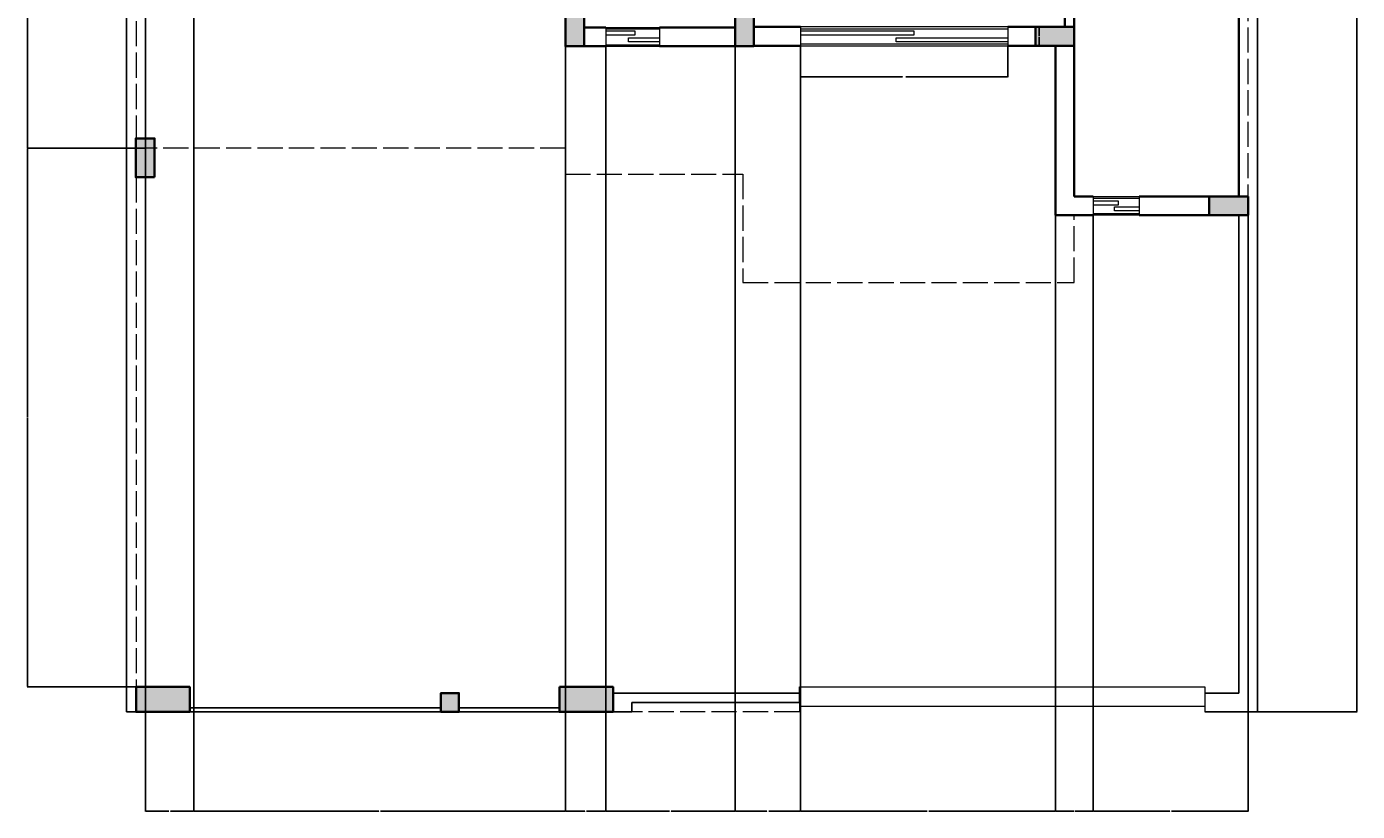
# Model space of a CAD drawing. Units: inches. Extents: x 2711 to 4246, y 540 to 1583.
# Tile 5 of 7: x 3610 to 4246, y 540 to 915. Entities that reach past the tile are written whole.
import ezdxf

# ---------------------------------------------------------------- set-up
doc = ezdxf.new("R2010")
doc.units = ezdxf.units.IN
doc.linetypes.add('ACAD_ISO02W100', pattern=[15, 12, -3])
for name, color, linetype, lineweight in [('A-ANNO-DIMS', 2, 'Continuous', 18), ('A-COLS', 210, 'Continuous', 35), ('A-COLS-PATT', 6, 'Continuous', 13), ('A-FLOR-OVHD', 225, 'ACAD_ISO02W100', 13), ('A-GLAZ', 4, 'Continuous', 18), ('A-WALL', 1, 'Continuous', 35), ('C-PROP-GATE', 32, 'Continuous', 18), ('C-PROP-HIDN', 7, 'ACAD_ISO02W100', 13), ('C-PROP-WALL', 7, 'Continuous', 25)]:
    doc.layers.add(name, color=color, linetype=linetype, lineweight=lineweight)
doc.styles.get("Standard").update_dxf_attribs({"font": 'arial.ttf'})
doc.dimstyles.get("Standard").update_dxf_attribs({"dimtxt": 0.18, "dimasz": 0.18, "dimexe": 0.18, "dimexo": 0.0625, "dimgap": 0.09, "dimtad": 0, "dimtih": 1, "dimtoh": 1, "dimdec": 4, "dimzin": 0, "dimdsep": 46, "dimtxsty": 'Standard', "dimcen": 0.09, "dimadec": 0, "dimazin": 0, "dimtfac": 1, "dimtdec": 4, "dimtofl": 0, "dimtmove": 0, "dimatfit": 3, "dimfxl": 1, "dimtolj": 1, "dimtzin": 0, "dimarcsym": 0})

# ---------------------------------------------------------------- blocks, each defined once
blk = doc.blocks.new('WIN-SLIDER-W02')
for p, q in [((0, 9), (0, 0)), ((0, 9), (25.68, 9)), ((0, 8.3), (25.68, 8.3)), ((0, 7.32), (13.85, 7.32)), ((13.85, 7.32), (13.85, 5.32)), ((25.68, 9), (25.68, 0)), ((13.85, 5.32), (0, 5.32)), ((0, 0.7), (25.68, 0.7)), ((10.83, 2.09), (10.83, 4.09)), ((10.83, 4.09), (25.68, 4.09)), ((25.68, 2.09), (10.83, 2.09)), ((0, 0), (25.68, 0))]:
    blk.add_line(p, q)
blk = doc.blocks.new('WIN-SLIDER-W03')
for p, q in [((0, 9), (0, 0)), ((99.07, 9), (0, 9)), ((0, 8.03), (99.07, 8.03)), ((0, 7.05), (54.2, 7.05)), ((54.2, 7.05), (54.2, 5.05)), ((99.07, 9), (99.07, 0)), ((54.2, 5.05), (0, 5.05)), ((0, 0.97), (99.07, 0.97)), ((45.64, 1.82), (45.64, 3.82)), ((45.64, 3.82), (99.07, 3.82)), ((99.07, 1.82), (45.64, 1.82)), ((0, 0), (99.07, 0))]:
    blk.add_line(p, q)
blk = doc.blocks.new('WIN-SLIDER-W04')
for p, q in [((0, 9), (0, 0)), ((0, 9), (22.02, 9)), ((0, 8.1), (22.02, 8.1)), ((0, 6.87), (11.87, 6.87)), ((11.87, 6.87), (11.87, 4.87)), ((22.02, 9), (22.02, 0)), ((11.87, 4.87), (0, 4.87)), ((0, 0.89), (22.02, 0.89)), ((10.15, 2.04), (10.15, 4.04)), ((10.15, 4.04), (22.02, 4.04)), ((22.02, 2.04), (10.15, 2.04)), ((22.02, 0), (0, 0))]:
    blk.add_line(p, q)
blk = doc.blocks.new('*D90')
at = {"layer": 'A-ANNO-DIMS', "color": 0, "lineweight": -2, "transparency": 16777216}
for p, q in [((3979.93, 905.71), (3979.93, 890.73)), ((4079, 905.71), (4079, 890.73)), ((3980.11, 890.91), (4028.64, 890.91)), ((4078.82, 890.91), (4030.29, 890.91))]:
    blk.add_line(p, q, dxfattribs=at)
at = {"layer": 'A-ANNO-DIMS', "color": 0, "transparency": 16777216}
for points in [[(3980.11, 890.94), (3980.11, 890.88), (3979.93, 890.91)], [(4078.82, 890.94), (4078.82, 890.88), (4079, 890.91)]]:
    blk.add_solid(points, dxfattribs=at)
at = {"layer": 'Defpoints', "color": 0, "transparency": 16777216}
for p in [(3979.93, 905.77), (4079, 905.77), (4079, 890.91)]:
    blk.add_point(p, dxfattribs=at)
at = {"layer": 'A-ANNO-DIMS', "color": 0, "transparency": 16777216, "insert": (4029.47, 890.91), "char_height": 0.18, "attachment_point": 5}
blk.add_mtext('\\A1;W03 99 TYP.', dxfattribs=at)
blk = doc.blocks.new('*D91')
at = {"layer": 'A-ANNO-DIMS', "color": 0, "lineweight": -2, "transparency": 16777216}
for p, q in [((4079.06, 914.77), (4094.04, 914.77)), ((4093.86, 914.59), (4093.86, 910.45)), ((4093.86, 905.95), (4093.86, 910.09)), ((4079.06, 905.77), (4094.04, 905.77))]:
    blk.add_line(p, q, dxfattribs=at)
at = {"layer": 'A-ANNO-DIMS', "color": 0, "transparency": 16777216}
for points in [[(4093.83, 914.59), (4093.89, 914.59), (4093.86, 914.77)], [(4093.83, 905.95), (4093.89, 905.95), (4093.86, 905.77)]]:
    blk.add_solid(points, dxfattribs=at)
at = {"layer": 'Defpoints', "color": 0, "transparency": 16777216}
for p in [(4079, 914.77), (4093.86, 914.77), (4079, 905.77)]:
    blk.add_point(p, dxfattribs=at)
at = {"layer": 'A-ANNO-DIMS', "color": 0, "transparency": 16777216, "insert": (4093.86, 910.27), "char_height": 0.18, "attachment_point": 5}
blk.add_mtext('\\A1;9 TYP.', dxfattribs=at)
blk = doc.blocks.new('*D97')
at = {"layer": 'A-ANNO-DIMS', "color": 0, "lineweight": -2, "transparency": 16777216}
for p, q in [((4198.24, 1534.95), (4245.74, 1534.95)), ((4245.56, 1534.77), (4245.56, 1061.38)), ((4245.56, 587.63), (4245.56, 1061.02)), ((4198.24, 587.45), (4245.74, 587.45))]:
    blk.add_line(p, q, dxfattribs=at)
at = {"layer": 'A-ANNO-DIMS', "color": 0, "transparency": 16777216}
for points in [[(4245.53, 1534.77), (4245.59, 1534.77), (4245.56, 1534.95)], [(4245.53, 587.63), (4245.59, 587.63), (4245.56, 587.45)]]:
    blk.add_solid(points, dxfattribs=at)
at = {"layer": 'Defpoints', "color": 0, "transparency": 16777216}
for p in [(4198.18, 1534.95), (4245.56, 1534.95), (4198.18, 587.45)]:
    blk.add_point(p, dxfattribs=at)
at = {"layer": 'A-ANNO-DIMS', "color": 0, "transparency": 16777216, "insert": (4245.56, 1061.2), "char_height": 0.18, "attachment_point": 5}
blk.add_mtext('\\A1;947.5', dxfattribs=at)
blk = doc.blocks.new('*D105')
at = {"layer": 'A-ANNO-DIMS', "color": 0, "lineweight": -2, "transparency": 16777216}
for p, q in [((3667.18, 1055.98), (3667.18, 539.89)), ((3690.29, 1055.1), (3690.29, 539.89)), ((3667.36, 540.07), (3678.36, 540.07)), ((3690.11, 540.07), (3679.12, 540.07))]:
    blk.add_line(p, q, dxfattribs=at)
at = {"layer": 'A-ANNO-DIMS', "color": 0, "transparency": 16777216}
for points in [[(3667.36, 540.1), (3667.36, 540.04), (3667.18, 540.07)], [(3690.11, 540.1), (3690.11, 540.04), (3690.29, 540.07)]]:
    blk.add_solid(points, dxfattribs=at)
at = {"layer": 'Defpoints', "color": 0, "transparency": 16777216}
for p in [(3667.18, 1056.04), (3690.29, 1055.17), (3690.29, 540.07)]:
    blk.add_point(p, dxfattribs=at)
at = {"layer": 'A-ANNO-DIMS', "color": 0, "transparency": 16777216, "insert": (3678.74, 540.07), "char_height": 0.18, "attachment_point": 5}
blk.add_mtext('\\A1;23.11', dxfattribs=at)
blk = doc.blocks.new('*D106')
at = {"layer": 'A-ANNO-DIMS', "color": 0, "lineweight": -2, "transparency": 16777216}
for p, q in [((3690.29, 1055.1), (3690.29, 539.89)), ((3867.71, 1046.98), (3867.71, 539.89)), ((3690.47, 540.07), (3778.62, 540.07)), ((3867.53, 540.07), (3779.39, 540.07))]:
    blk.add_line(p, q, dxfattribs=at)
at = {"layer": 'A-ANNO-DIMS', "color": 0, "transparency": 16777216}
for points in [[(3690.47, 540.1), (3690.47, 540.04), (3690.29, 540.07)], [(3867.53, 540.1), (3867.53, 540.04), (3867.71, 540.07)]]:
    blk.add_solid(points, dxfattribs=at)
at = {"layer": 'Defpoints', "color": 0, "transparency": 16777216}
for p in [(3690.29, 1055.17), (3867.71, 1047.04), (3867.71, 540.07)]:
    blk.add_point(p, dxfattribs=at)
at = {"layer": 'A-ANNO-DIMS', "color": 0, "transparency": 16777216, "insert": (3779, 540.07), "char_height": 0.18, "attachment_point": 5}
blk.add_mtext('\\A1;177.4', dxfattribs=at)
blk = doc.blocks.new('*D107')
at = {"layer": 'A-ANNO-DIMS', "color": 0, "lineweight": -2, "transparency": 16777216}
for p, q in [((3867.71, 905.43), (3867.71, 539.89)), ((3887.03, 905.43), (3887.03, 539.89)), ((3867.89, 540.07), (3876.98, 540.07)), ((3886.85, 540.07), (3877.75, 540.07))]:
    blk.add_line(p, q, dxfattribs=at)
at = {"layer": 'A-ANNO-DIMS', "color": 0, "transparency": 16777216}
for points in [[(3867.89, 540.1), (3867.89, 540.04), (3867.71, 540.07)], [(3886.85, 540.1), (3886.85, 540.04), (3887.03, 540.07)]]:
    blk.add_solid(points, dxfattribs=at)
at = {"layer": 'Defpoints', "color": 0, "transparency": 16777216}
for p in [(3867.71, 905.5), (3887.03, 905.5), (3887.03, 540.07)]:
    blk.add_point(p, dxfattribs=at)
at = {"layer": 'A-ANNO-DIMS', "color": 0, "transparency": 16777216, "insert": (3877.37, 540.07), "char_height": 0.18, "attachment_point": 5}
blk.add_mtext('\\A1;19.32', dxfattribs=at)
blk = doc.blocks.new('*D108')
at = {"layer": 'A-ANNO-DIMS', "color": 0, "lineweight": -2, "transparency": 16777216}
for p, q in [((3887.03, 905.43), (3887.03, 539.89)), ((3948.71, 905.43), (3948.71, 539.89)), ((3887.21, 540.07), (3917.47, 540.07)), ((3948.53, 540.07), (3918.26, 540.07))]:
    blk.add_line(p, q, dxfattribs=at)
at = {"layer": 'A-ANNO-DIMS', "color": 0, "transparency": 16777216}
for points in [[(3887.21, 540.1), (3887.21, 540.04), (3887.03, 540.07)], [(3948.53, 540.1), (3948.53, 540.04), (3948.71, 540.07)]]:
    blk.add_solid(points, dxfattribs=at)
at = {"layer": 'Defpoints', "color": 0, "transparency": 16777216}
for p in [(3887.03, 905.5), (3948.71, 905.5), (3948.71, 540.07)]:
    blk.add_point(p, dxfattribs=at)
at = {"layer": 'A-ANNO-DIMS', "color": 0, "transparency": 16777216, "insert": (3917.87, 540.07), "char_height": 0.18, "attachment_point": 5}
blk.add_mtext('\\A1;61.68', dxfattribs=at)
blk = doc.blocks.new('*D109')
at = {"layer": 'A-ANNO-DIMS', "color": 0, "lineweight": -2, "transparency": 16777216}
for p, q in [((3948.71, 905.43), (3948.71, 539.89)), ((3979.93, 905.71), (3979.93, 539.89)), ((3948.89, 540.07), (3963.86, 540.07)), ((3979.75, 540.07), (3964.78, 540.07))]:
    blk.add_line(p, q, dxfattribs=at)
at = {"layer": 'A-ANNO-DIMS', "color": 0, "transparency": 16777216}
for points in [[(3948.89, 540.1), (3948.89, 540.04), (3948.71, 540.07)], [(3979.75, 540.1), (3979.75, 540.04), (3979.93, 540.07)]]:
    blk.add_solid(points, dxfattribs=at)
at = {"layer": 'Defpoints', "color": 0, "transparency": 16777216}
for p in [(3948.71, 905.5), (3979.93, 905.77), (3979.93, 540.07)]:
    blk.add_point(p, dxfattribs=at)
at = {"layer": 'A-ANNO-DIMS', "color": 0, "transparency": 16777216, "insert": (3964.32, 540.07), "char_height": 0.18, "attachment_point": 5}
blk.add_mtext('\\A1;31.226', dxfattribs=at)
blk = doc.blocks.new('*D110')
at = {"layer": 'A-ANNO-DIMS', "color": 0, "lineweight": -2, "transparency": 16777216}
for p, q in [((3979.93, 905.71), (3979.93, 539.89)), ((4101.71, 905.71), (4101.71, 539.89)), ((3980.11, 540.07), (4040.36, 540.07)), ((4101.53, 540.07), (4041.28, 540.07))]:
    blk.add_line(p, q, dxfattribs=at)
at = {"layer": 'A-ANNO-DIMS', "color": 0, "transparency": 16777216}
for points in [[(3980.11, 540.1), (3980.11, 540.04), (3979.93, 540.07)], [(4101.53, 540.1), (4101.53, 540.04), (4101.71, 540.07)]]:
    blk.add_solid(points, dxfattribs=at)
at = {"layer": 'Defpoints', "color": 0, "transparency": 16777216}
for p in [(3979.93, 905.77), (4101.71, 905.77), (4101.71, 540.07)]:
    blk.add_point(p, dxfattribs=at)
at = {"layer": 'A-ANNO-DIMS', "color": 0, "transparency": 16777216, "insert": (4040.82, 540.07), "char_height": 0.18, "attachment_point": 5}
blk.add_mtext('\\A1;121.77', dxfattribs=at)
blk = doc.blocks.new('*D111')
at = {"layer": 'A-ANNO-DIMS', "color": 0, "lineweight": -2, "transparency": 16777216}
for p, q in [((4101.71, 824.71), (4101.71, 539.89)), ((4119.71, 824.71), (4119.71, 539.89)), ((4101.89, 540.07), (4110.5, 540.07)), ((4119.53, 540.07), (4110.92, 540.07))]:
    blk.add_line(p, q, dxfattribs=at)
at = {"layer": 'A-ANNO-DIMS', "color": 0, "transparency": 16777216}
for points in [[(4101.89, 540.1), (4101.89, 540.04), (4101.71, 540.07)], [(4119.53, 540.1), (4119.53, 540.04), (4119.71, 540.07)]]:
    blk.add_solid(points, dxfattribs=at)
at = {"layer": 'Defpoints', "color": 0, "transparency": 16777216}
for p in [(4101.71, 824.77), (4119.71, 824.77), (4119.71, 540.07)]:
    blk.add_point(p, dxfattribs=at)
at = {"layer": 'A-ANNO-DIMS', "color": 0, "transparency": 16777216, "insert": (4110.71, 540.07), "char_height": 0.18, "attachment_point": 5}
blk.add_mtext('\\A1;18', dxfattribs=at)
blk = doc.blocks.new('*D112')
at = {"layer": 'A-ANNO-DIMS', "color": 0, "lineweight": -2, "transparency": 16777216}
for p, q in [((4119.71, 824.71), (4119.71, 539.89)), ((4193.68, 824.69), (4193.68, 539.89)), ((4119.89, 540.07), (4156.3, 540.07)), ((4193.5, 540.07), (4157.09, 540.07))]:
    blk.add_line(p, q, dxfattribs=at)
at = {"layer": 'A-ANNO-DIMS', "color": 0, "transparency": 16777216}
for points in [[(4119.89, 540.1), (4119.89, 540.04), (4119.71, 540.07)], [(4193.5, 540.1), (4193.5, 540.04), (4193.68, 540.07)]]:
    blk.add_solid(points, dxfattribs=at)
at = {"layer": 'Defpoints', "color": 0, "transparency": 16777216}
for p in [(4119.71, 824.77), (4193.68, 824.75), (4193.68, 540.07)]:
    blk.add_point(p, dxfattribs=at)
at = {"layer": 'A-ANNO-DIMS', "color": 0, "transparency": 16777216, "insert": (4156.69, 540.07), "char_height": 0.18, "attachment_point": 5}
blk.add_mtext('\\A1;73.97', dxfattribs=at)
blk = doc.blocks.new('*D124')
at = {"layer": 'A-ANNO-DIMS', "color": 0, "lineweight": -2, "transparency": 16777216}
for p, q in [((3666.97, 856.87), (3610.62, 856.87)), ((3610.8, 856.69), (3610.8, 728.3)), ((3610.8, 599.54), (3610.8, 727.93)), ((3667.12, 599.36), (3610.62, 599.36))]:
    blk.add_line(p, q, dxfattribs=at)
at = {"layer": 'A-ANNO-DIMS', "color": 0, "transparency": 16777216}
for points in [[(3610.77, 856.69), (3610.83, 856.69), (3610.8, 856.87)], [(3610.77, 599.54), (3610.83, 599.54), (3610.8, 599.36)]]:
    blk.add_solid(points, dxfattribs=at)
at = {"layer": 'Defpoints', "color": 0, "transparency": 16777216}
for p in [(3610.8, 856.87), (3667.03, 856.87), (3667.18, 599.36)]:
    blk.add_point(p, dxfattribs=at)
at = {"layer": 'A-ANNO-DIMS', "color": 0, "transparency": 16777216, "insert": (3610.8, 728.12), "char_height": 0.18, "attachment_point": 5}
blk.add_mtext('\\A1;257.5', dxfattribs=at)
blk = doc.blocks.new('*D125')
at = {"layer": 'A-ANNO-DIMS', "color": 0, "lineweight": -2, "transparency": 16777216}
for p, q in [((3671.47, 1047.04), (3610.62, 1047.04)), ((3610.8, 1046.86), (3610.8, 952.14)), ((3610.8, 857.05), (3610.8, 951.78)), ((3666.97, 856.87), (3610.62, 856.87))]:
    blk.add_line(p, q, dxfattribs=at)
at = {"layer": 'A-ANNO-DIMS', "color": 0, "transparency": 16777216}
for points in [[(3610.77, 1046.86), (3610.83, 1046.86), (3610.8, 1047.04)], [(3610.77, 857.05), (3610.83, 857.05), (3610.8, 856.87)]]:
    blk.add_solid(points, dxfattribs=at)
at = {"layer": 'Defpoints', "color": 0, "transparency": 16777216}
for p in [(3610.8, 1047.04), (3671.53, 1047.04), (3667.03, 856.87)]:
    blk.add_point(p, dxfattribs=at)
at = {"layer": 'A-ANNO-DIMS', "color": 0, "transparency": 16777216, "insert": (3610.8, 951.96), "char_height": 0.18, "attachment_point": 5}
blk.add_mtext('\\A1;190.16', dxfattribs=at)

msp = doc.modelspace()

# ---------------------------------------------------------------- hatches: boundary and pattern name
at = {"layer": 'A-COLS-PATT'}
h = msp.add_hatch(color=256, dxfattribs=at)
h.dxf.hatch_style = 1
h.paths.add_polyline_path([(3662.6812, 1384.9055), (3671.6812, 1384.9055), (3671.6812, 1403.4493), (3662.6812, 1403.4493)])
h.paths.add_polyline_path([(3960.225, 1394.4493), (3960.225, 1403.4493), (3941.6812, 1403.4493), (3941.6812, 1394.4493)])
h.paths.add_polyline_path([(4193.6812, 1394.4493), (4193.6812, 1403.4493), (4175.1375, 1403.4493), (4175.1375, 1394.4493)])
h.paths.add_polyline_path([(3662.5342, 1230.0438), (3671.5342, 1230.0353), (3671.5342, 1248.5791), (3662.5342, 1248.5791)])
h.paths.add_polyline_path([(3766.6812, 1229.9493), (3766.6812, 1238.9493), (3758.128, 1238.9493), (3758.128, 1229.9531), (3762.1812, 1229.9493)])
h.paths.add_polyline_path([(3950.6812, 1229.9493), (3950.6812, 1238.9493), (3932.1375, 1238.9493), (3932.1375, 1229.9493)])
h.paths.add_polyline_path([(4193.6812, 1229.9493), (4193.6812, 1238.9493), (4175.1375, 1238.9493), (4175.1375, 1229.9493)])
h.paths.add_polyline_path([(3671.5342, 1056.0394), (3662.5342, 1056.0394), (3662.5342, 1037.4957), (3671.5342, 1037.4957)])
h.paths.add_polyline_path([(3867.7072, 1041.7894), (3867.7072, 1037.4957), (3876.7006, 1037.4957), (3876.7006, 1056.0394), (3867.7006, 1056.0394), (3867.7006, 1052.2894), (3867.7072, 1052.2894), (3867.7072, 1047.0394)])
h.paths.add_polyline_path([(3957.7072, 1037.4957), (3957.7072, 1056.0394), (3948.7072, 1056.0394), (3948.7072, 1037.4957)])
h.paths.add_polyline_path([(4189.1812, 1046.9493), (4193.6812, 1046.9493), (4193.6812, 1055.9413), (4175.1375, 1055.9413), (4175.1375, 1046.9493)])
h.paths.add_polyline_path([(3876.7072, 924.0394), (3867.7072, 924.0394), (3867.7072, 905.4957), (3876.7072, 905.4957)])
h.paths.add_polyline_path([(3948.7072, 905.4957), (3957.7072, 905.4957), (3957.7072, 924.0394), (3948.7072, 924.0394)])
h.paths.add_polyline_path([(4110.7072, 905.7675), (4110.7072, 914.7675), (4092.1634, 914.7675), (4092.1634, 905.7675)])
h.paths.add_polyline_path([(3671.5342, 842.8947), (3671.5342, 861.4385), (3662.5342, 861.4385), (3662.5342, 842.8947)])
h.paths.add_polyline_path([(4189.1812, 824.7675), (4193.6812, 824.7498), (4193.6812, 833.7498), (4175.1375, 833.7498), (4175.1375, 824.7675)])
h.paths.add_polyline_path([(3688.2903, 587.4493), (3688.2903, 599.3563), (3662.6812, 599.3563), (3662.6812, 587.4493)])
h.paths.add_polyline_path([(3816.8435, 587.4493), (3816.8435, 596.4493), (3808.2903, 596.4493), (3808.2903, 587.4493)])
h.paths.add_polyline_path([(3890.4526, 587.4493), (3890.4526, 599.3563), (3864.8435, 599.3563), (3864.8435, 587.4493)])

# ---------------------------------------------------------------- linework, layer by layer
at = {"layer": 'A-COLS'}
msp.add_line((3816.8435, 596.4493), (3808.2903, 596.4493), dxfattribs=at)
for points in [[(3876.7072, 905.4957), (3876.7072, 924.0394), (3867.7072, 924.0394), (3867.7072, 905.4957)], [(3957.7072, 905.4957), (3957.7072, 924.0394), (3948.7072, 924.0394), (3948.7072, 905.4957)], [(4110.7072, 914.7675), (4092.1634, 914.7675), (4092.1634, 905.7675), (4110.7072, 905.7675)], [(3671.5342, 842.8947), (3671.5342, 861.4385), (3662.5342, 861.4385), (3662.5342, 842.8947)], [(4193.6812, 833.7498), (4175.1375, 833.7498), (4175.1375, 824.7498), (4193.6812, 824.7498)], [(3662.6812, 599.3563), (3688.2903, 599.3563), (3688.2903, 587.4493), (3662.6812, 587.4493)], [(3864.8435, 599.3563), (3890.4526, 599.3563), (3890.4526, 587.4493), (3864.8435, 587.4493)], [(3808.2903, 587.4493), (3816.8435, 587.4493), (3816.8435, 596.4493), (3808.2903, 596.4493)]]:
    msp.add_lwpolyline(points, close=True, dxfattribs=at)
at = {"layer": 'A-FLOR-OVHD'}
for p, q in [((3867.7072, 905.4957), (3867.7072, 844.38)), ((3867.7072, 856.8749), (3667.0342, 856.8749)), ((3867.7072, 844.38), (3952.4813, 844.38)), ((3952.4813, 844.38), (3952.4813, 792.5892)), ((4110.7072, 792.5892), (4110.7072, 824.7675)), ((3952.4813, 792.5892), (4110.7072, 792.5892))]:
    msp.add_line(p, q, dxfattribs=at)
at = {"layer": 'A-WALL'}
for p, q in [((4189.1812, 1046.9493), (4189.1812, 833.7498)), ((4106.2072, 1016.0126), (4106.2072, 914.7675)), ((4110.7072, 914.7675), (4110.7072, 1016.0126)), ((3887.0265, 914.4957), (3876.7072, 914.4957)), ((3948.7072, 914.4957), (3912.7072, 914.4957)), ((3957.7072, 914.7675), (3979.9331, 914.7675)), ((3957.7072, 905.7675), (3957.7072, 914.7675)), ((4078.9994, 914.7675), (4110.7072, 914.7675)), ((4110.7072, 914.7675), (4110.7072, 905.7675)), ((3876.7072, 905.4957), (3887.0265, 905.4957)), ((3912.7072, 905.4957), (3948.7072, 905.4957)), ((3979.9331, 905.7675), (3957.7072, 905.7675)), ((4110.7072, 905.7675), (4078.9994, 905.7675)), ((4101.7072, 824.7675), (4101.7072, 905.7675)), ((4110.7072, 905.7675), (4110.7072, 833.7675)), ((4110.7072, 833.7675), (4119.7072, 833.7675)), ((4141.7223, 833.7675), (4189.1812, 833.7675)), ((4110.7072, 824.7675), (4101.7072, 824.7675)), ((4119.7072, 824.7675), (4110.7072, 824.7675)), ((4141.7223, 824.7675), (4189.1812, 824.7675))]:
    msp.add_line(p, q, dxfattribs=at)
at = {"layer": 'C-PROP-GATE'}
for p, q in [((3979.4526, 596.4493), (3979.4526, 599.4493)), ((3979.4526, 599.4493), (4173.1007, 599.4493)), ((4173.1007, 599.4493), (4173.1007, 596.4493)), ((3979.4526, 591.9493), (3979.4526, 596.4493)), ((3979.4526, 591.9493), (3979.4526, 596.4493)), ((3979.4526, 591.9493), (3979.4526, 589.9493)), ((4173.1007, 596.4493), (4173.1007, 591.9493)), ((4173.1007, 591.9493), (4173.1007, 589.9493)), ((4173.1007, 589.9493), (3979.4526, 589.9493)), ((3979.4526, 589.9493), (3979.4526, 587.4493)), ((4173.1007, 589.9493), (4173.1007, 587.4493))]:
    msp.add_line(p, q, dxfattribs=at)
at = {"layer": 'C-PROP-HIDN'}
for p, q in [((4193.6812, 587.4493), (4193.6812, 1530.4493)), ((3662.6812, 1037.4957), (3662.6812, 861.4385)), ((3662.6812, 842.8947), (3662.6812, 587.4493)), ((3979.4526, 591.9493), (3979.4526, 596.4493)), ((3979.4526, 587.4493), (3899.4526, 587.4493))]:
    msp.add_line(p, q, dxfattribs=at)
at = {"layer": 'C-PROP-WALL'}
for p, q in [((3658.1812, 587.4493), (3658.1812, 1530.4493)), ((4198.1812, 1530.4493), (4198.1812, 587.4493)), ((3667.1812, 861.4385), (3667.1812, 1037.4957)), ((3667.1812, 599.3563), (3667.1812, 842.8947)), ((4189.1812, 824.7675), (4189.1812, 596.4493)), ((3979.4526, 596.4493), (3890.4526, 596.4493)), ((3899.4526, 587.4493), (3899.4526, 591.9493)), ((3899.4526, 591.9493), (3979.4526, 591.9493)), ((4189.1812, 596.4493), (4173.1007, 596.4493)), ((3662.6812, 587.4493), (3658.1812, 587.4493)), ((3688.2903, 589.4493), (3808.2903, 589.4493)), ((3688.2903, 587.4493), (3808.2903, 587.4493)), ((3808.2903, 589.4493), (3808.2903, 587.4493)), ((3816.8435, 589.4493), (3864.8435, 589.4493)), ((3816.8435, 587.4493), (3864.8435, 587.4493)), ((3864.8435, 589.4493), (3864.8435, 587.4493)), ((3890.4526, 587.4493), (3893.4526, 587.4493)), ((3893.4526, 587.4493), (3895.4526, 587.4493)), ((3895.4526, 587.4493), (3897.4526, 587.4493)), ((3897.4526, 587.4493), (3899.4526, 587.4493)), ((4193.6812, 587.4493), (4173.1007, 587.4493)), ((4198.1812, 587.4493), (4193.6812, 587.4493))]:
    msp.add_line(p, q, dxfattribs=at)

# ---------------------------------------------------------------- block references
at = {"layer": 'A-GLAZ'}
for name, p in [('WIN-SLIDER-W02', (3887.0268, 905.496)), ('WIN-SLIDER-W03', (3979.9328, 905.768)), ('WIN-SLIDER-W04', (4119.7068, 824.768))]:
    msp.add_blockref(name, p, dxfattribs=at)

# ---------------------------------------------------------------- dimensions: what is measured, and where the dimension line sits
at = {"layer": 'A-ANNO-DIMS'}
for base, p1, p2, override, picture, middle in [((4245.5582, 1534.9493), (4198.1812, 587.4493), (4198.1812, 1534.9493), {"dimdec": 1, "dimlfac": 1, "dimrnd": 0, "dimzin": 0, "dimdsep": 46, "dimlunit": 2}, '*D97', (4245.5582, 1061.1993)), ((3610.8042, 1047.0394), (3667.0342, 856.8749), (3671.5342, 1047.0394), {"dimdec": 2, "dimlfac": 1, "dimrnd": 0, "dimzin": 0, "dimdsep": 46, "dimlunit": 2}, '*D125', (3610.8042, 951.9572)), ((3610.8042, 856.8749), (3667.1812, 599.3563), (3667.0342, 856.8749), {"dimdec": 1, "dimlfac": 1, "dimrnd": 0, "dimzin": 0, "dimdsep": 46, "dimlunit": 2}, '*D124', (3610.8042, 728.1156))]:
    dim = msp.add_linear_dim(base=base, p1=p1, p2=p2, angle=90, dimstyle='Standard', override=override, dxfattribs=at)
    dim.commit()
    dim.dimension.update_dxf_attribs({"geometry": picture, "text_midpoint": middle})
for base, p1, p2, override, picture, middle in [((3690.2931, 540.0723), (3667.1812, 1056.0394), (3690.2931, 1055.1667), {"dimdec": 2, "dimlfac": 1, "dimrnd": 0, "dimzin": 0, "dimdsep": 46, "dimlunit": 2}, '*D105', (3678.7372, 540.0723)), ((3867.7072, 540.0723), (3690.2931, 1055.1667), (3867.7072, 1047.0394), {"dimdec": 1, "dimlfac": 1, "dimrnd": 0, "dimzin": 0, "dimdsep": 46, "dimlunit": 2}, '*D106', (3779.0001, 540.0723)), ((3887.0265, 540.0723), (3867.7072, 905.4957), (3887.0265, 905.4957), {"dimdec": 2, "dimlfac": 1, "dimrnd": 0, "dimzin": 0, "dimdsep": 46, "dimlunit": 2}, '*D107', (3877.3668, 540.0723)), ((3948.7072, 540.0723), (3887.0265, 905.4957), (3948.7072, 905.4957), {"dimdec": 2, "dimlfac": 1, "dimrnd": 0, "dimzin": 0, "dimdsep": 46, "dimlunit": 2}, '*D108', (3917.8668, 540.0723)), ((3979.9331, 540.0723), (3948.7072, 905.4957), (3979.9331, 905.7675), {"dimdec": 3, "dimlfac": 1, "dimrnd": 0, "dimzin": 0, "dimdsep": 46, "dimlunit": 2}, '*D109', (3964.3201, 540.0723)), ((4101.7072, 540.0723), (3979.9331, 905.7675), (4101.7072, 905.7675), {"dimdec": 2, "dimlfac": 1, "dimrnd": 0, "dimzin": 0, "dimdsep": 46, "dimlunit": 2}, '*D110', (4040.8201, 540.0723)), ((4119.7072, 540.0723), (4101.7072, 824.7675), (4119.7072, 824.7675), {"dimdec": 0, "dimlfac": 1, "dimrnd": 0, "dimzin": 0, "dimdsep": 46, "dimlunit": 2}, '*D111', (4110.7072, 540.0723)), ((4193.6812, 540.0723), (4119.7072, 824.7675), (4193.6812, 824.7498), {"dimdec": 2, "dimlfac": 1, "dimrnd": 0, "dimzin": 0, "dimdsep": 46, "dimlunit": 2}, '*D112', (4156.6942, 540.0723))]:
    dim = msp.add_linear_dim(base=base, p1=p1, p2=p2, dimstyle='Standard', override=override, dxfattribs=at)
    dim.commit()
    dim.dimension.update_dxf_attribs({"geometry": picture, "text_midpoint": middle})
dim = msp.add_linear_dim(base=(4093.8593, 914.7675), p1=(4078.9994, 905.7675), p2=(4078.9994, 914.7675), angle=90, text='<> TYP.', dimstyle='Standard', override={"dimdec": 0, "dimlfac": 1, "dimrnd": 0, "dimzin": 0, "dimdsep": 46, "dimlunit": 2}, dxfattribs=at)
dim.commit()
dim.dimension.update_dxf_attribs({"geometry": '*D91', "text_midpoint": (4093.8593, 910.2675)})
dim = msp.add_linear_dim(base=(4078.9994, 890.9076), p1=(3979.9331, 905.7675), p2=(4078.9994, 905.7675), text='W03 <> TYP.', dimstyle='Standard', override={"dimdec": 0, "dimlfac": 1, "dimrnd": 0, "dimzin": 0, "dimdsep": 46, "dimlunit": 2}, dxfattribs=at)
dim.commit()
dim.dimension.update_dxf_attribs({"geometry": '*D90', "text_midpoint": (4029.4662, 890.9076)})

doc.saveas('drawing.dxf')
